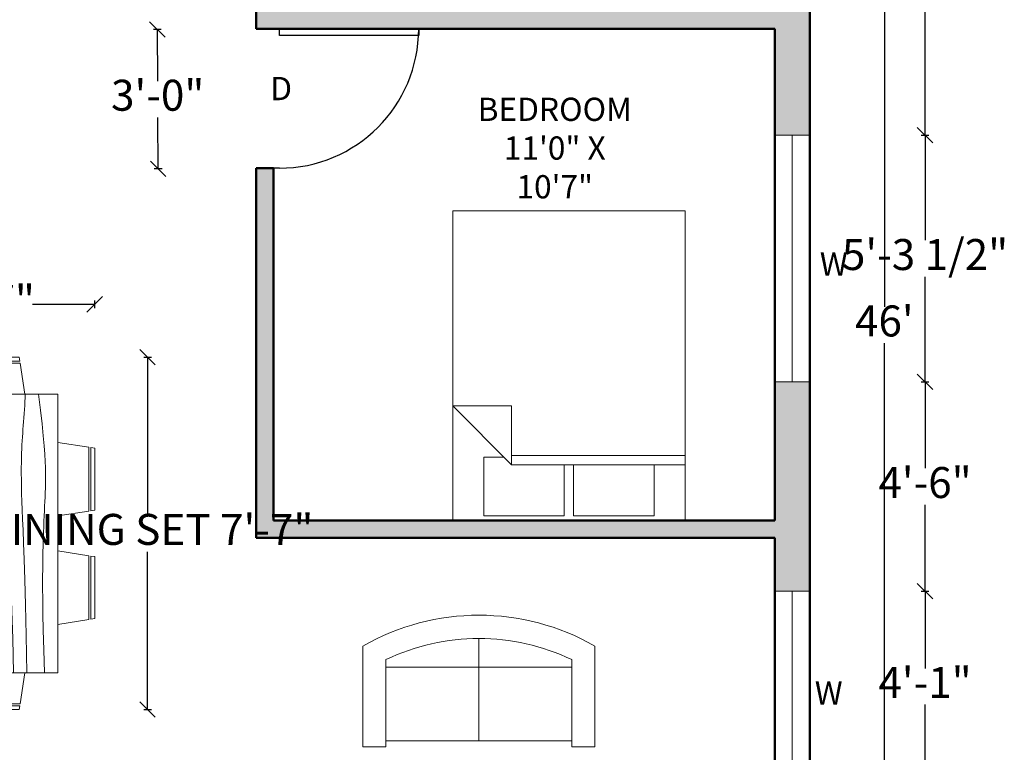
# Model space of a CAD drawing. Units: inches. Extents: x 2395 to 2921, y 528 to 1164.
# Tile 4 of 5: x 2662 to 2916, y 735 to 925. Entities that reach past the tile are written whole.
import ezdxf

# ---------------------------------------------------------------- set-up
doc = ezdxf.new("R2010")
doc.units = ezdxf.units.IN
for name, color, linetype, lineweight in [('A-ANNO-DIMS', 2, 'Continuous', 18), ('A-ANNO-TEXT', 7, 'Continuous', 18), ('A-AREA-IDEN', 7, 'Continuous', 25), ('A-DOOR', 3, 'Continuous', 25), ('A-FURN', 8, 'Continuous', 18), ('A-GLAZ', 4, 'Continuous', 18), ('A-WALL', 162, 'Continuous', 50), ('A-WALL-PATT', 162, 'Continuous', 13)]:
    doc.layers.add(name, color=color, linetype=linetype, lineweight=lineweight)
doc.styles.get("Standard").update_dxf_attribs({"font": 'arial.ttf'})
doc.dimstyles.new('ISO-25', dxfattribs={"dimtxt": 8, "dimasz": 4, "dimexe": 1, "dimexo": 1, "dimtad": 0, "dimtih": 1, "dimtoh": 1, "dimlunit": 3, "dimtxsty": 'Standard', "dimblk": 'OBLIQUE', "dimcen": 2.5, "dimadec": 0, "dimazin": 0, "dimtfac": 1, "dimtmove": 0, "dimatfit": 3, "dimfxl": 1, "dimfxlon": 1, "dimarcsym": 0})

# ---------------------------------------------------------------- blocks, each defined once
blk = doc.blocks.new('*U7')
for p, q in [((0, 0), (0, -6)), ((36, 0), (36, -6))]:
    blk.add_line(p, q)
blk.add_lwpolyline([(0, 0), (0, 36), (1.75, 36), (1.75, 0)], close=True)
blk.add_arc((0, 0), 36, 0, 90)
blk = doc.blocks.new('Sofa - Roundback Loveseat 5 ft.')
for p, q in [((0, -32.44198), (0, -5.99998)), ((-24, -33.99998), (-24, -11.46958)), ((24.00004, -33.99998), (24.00004, -11.46958)), ((-23.9998, -13.38178), (23.99986, -13.38178)), ((-24, -32.44198), (24.00004, -32.44198))]:
    blk.add_line(p, q)
for points in [[(-24, -33.99998), (-30, -33.99998), (-30, -7.99998)], [(30.00004, -7.99998), (30.00004, -33.99998), (24.00004, -33.99998)]]:
    blk.add_lwpolyline(points)
for centre, radius, start, end in [((0, -60.24998), 60.24998, 60.13715, 119.8628), ((0, -61.38438), 55.38444, 64.32083, 115.6792)]:
    blk.add_arc(centre, radius, start, end)
blk = doc.blocks.new('Dining Set - 36 x 72 in.')
for p, q in [((-22.2343, 26.00059), (-23.4847, 17.99762)), ((-22.2304, 26), (-5.7608, 26)), ((-22, 27.5), (-22.1562, 26.50042)), ((-5.8416, 26.5), (-22.1534, 26.5)), ((-22, 27.5), (-6, 27.5)), ((-5.8437, 26.49966), (-6, 27.5)), ((-4.5152, 17.99762), (-5.7655, 25.99926)), ((5.7657, 26.00059), (4.5153, 17.99762)), ((5.7696, 26), (22.2392, 26)), ((6, 27.5), (5.8438, 26.50042)), ((22.1584, 26.5), (5.8466, 26.5)), ((6, 27.5), (22, 27.5)), ((22.1563, 26.49966), (22, 27.5)), ((23.4848, 17.99762), (22.2345, 25.99926)), ((36, 18), (-36, 18)), ((-36, 18), (-36, -18)), ((36, -18), (36, 18)), ((-45.5, 8), (-44.5004, 8.15617)), ((-45.5, 8), (-45.5, -8)), ((-44.5, -8.15843), (-44.5, 8.15338)), ((-44.0006, 8.23428), (-35.9976, 9.48474)), ((-44, 8.23041), (-44, -8.23915)), ((44.0006, 8.23428), (35.9976, 9.48474)), ((44, 8.23041), (44, -8.23915)), ((44.5, -8.15843), (44.5, 8.15338)), ((45.5, 8), (44.5005, 8.15617)), ((45.5, 8), (45.5, -8)), ((-44.4997, -8.15631), (-45.5, -8)), ((-35.9976, -9.48476), (-43.9993, -8.2345)), ((35.9976, -9.48476), (43.9993, -8.2345)), ((44.4997, -8.15631), (45.5, -8)), ((-36, -18), (36, -18)), ((-22.2343, -26.0006), (-23.4847, -17.99762)), ((-4.5152, -17.99762), (-5.7655, -25.99928)), ((5.7657, -26.0006), (4.5153, -17.99762)), ((23.4848, -17.99762), (22.2345, -25.99928)), ((-22.2304, -26), (-5.7608, -26)), ((-22, -27.5), (-22.1562, -26.50044)), ((-5.8416, -26.5), (-22.1534, -26.5)), ((-22, -27.5), (-6, -27.5)), ((-5.8437, -26.49967), (-6, -27.5)), ((5.7696, -26), (22.2392, -26)), ((6, -27.5), (5.8438, -26.50044)), ((22.1584, -26.5), (5.8466, -26.5)), ((6, -27.5), (22, -27.5)), ((22.1563, -26.49967), (22, -27.5))]:
    blk.add_line(p, q)
for points in [[(-36, 15), (-31.1772, 14.97754), (-26.8079, 14.91406), (-22.8538, 14.81543), (-19.276, 14.6875), (-16.0362, 14.53613), (-13.0957, 14.36718), (-10.4159, 14.18652), (-7.9583, 14), (-5.6904, 13.81315), (-3.6035, 13.63021), (-1.6954, 13.45508), (0.0365, 13.29166), (1.5945, 13.14388), (2.9811, 13.01562), (4.1988, 12.9108), (5.25, 12.83333), (6.1393, 12.78613), (6.8802, 12.76823), (7.4883, 12.77767), (7.9792, 12.8125), (8.3685, 12.87077), (8.6719, 12.95052), (8.9049, 13.0498), (9.0833, 13.16666), (9.2205, 13.29899), (9.3216, 13.44401), (9.3895, 13.59879), (9.4271, 13.76041), (9.4373, 13.92594), (9.4232, 14.09245), (9.3875, 14.257), (9.3333, 14.41666), (9.2638, 14.56917), (9.1836, 14.71484), (9.0975, 14.85465), (9.0104, 14.98958), (8.9272, 15.1206), (8.8529, 15.2487), (8.7922, 15.37483), (8.75, 15.5), (8.7305, 15.62467), (8.7344, 15.74739), (8.7617, 15.86621), (8.8125, 15.97916), (8.8867, 16.08431), (8.9844, 16.17968), (9.1055, 16.26334), (9.25, 16.33333), (9.4189, 16.38802), (9.6172, 16.42708), (9.8506, 16.45052), (10.125, 16.45833), (10.4463, 16.45052), (10.8203, 16.42708), (11.2529, 16.38802), (11.75, 16.33333), (12.3184, 16.26318), (12.9694, 16.17838), (13.7151, 16.07991), (14.5677, 15.96875), (15.5395, 15.84586), (16.6426, 15.71224), (17.8893, 15.56884), (19.2917, 15.41666), (20.859, 15.25667), (22.5879, 15.08984), (24.4721, 14.91715), (26.5052, 14.73958), (28.6809, 14.5581), (30.9929, 14.3737), (33.4347, 14.18733), (36, 14)], [(-36, 10), (-28.9766, 10.14274), (-23.1725, 10.20442), (-18.4241, 10.19775), (-14.5677, 10.13541), (-11.4399, 10.03011), (-8.877, 9.89453), (-6.7154, 9.74137), (-4.7917, 9.58333), (-2.9698, 9.43082), (-1.2246, 9.28515), (0.4415, 9.14534), (2.026, 9.01041), (3.5266, 8.87939), (4.9408, 8.7513), (6.266, 8.62516), (7.5, 8.5), (8.6411, 8.37549), (9.6914, 8.2539), (10.6538, 8.13818), (11.5312, 8.03125), (12.3267, 7.93603), (13.043, 7.85547), (13.6831, 7.79248), (14.25, 7.75), (14.7471, 7.7303), (15.1797, 7.73307), (15.5537, 7.75732), (15.875, 7.80208), (16.1494, 7.86637), (16.3828, 7.94922), (16.5811, 8.04964), (16.75, 8.16666), (16.8944, 8.29915), (17.0143, 8.44531), (17.1089, 8.60319), (17.1771, 8.77083), (17.218, 8.94629), (17.2305, 9.1276), (17.2137, 9.31282), (17.1667, 9.5), (17.0895, 9.6875), (16.987, 9.875), (16.8649, 10.0625), (16.7292, 10.25), (16.5856, 10.4375), (16.4401, 10.625), (16.2985, 10.8125), (16.1667, 11), (16.05, 11.18733), (15.9518, 11.3737), (15.8752, 11.5581), (15.8229, 11.73958), (15.798, 11.91715), (15.8034, 12.08984), (15.842, 12.25667), (15.9167, 12.41666), (16.0295, 12.56836), (16.1784, 12.70833), (16.3605, 12.83268), (16.5729, 12.9375), (16.8127, 13.01888), (17.0768, 13.07291), (17.3625, 13.0957), (17.6667, 13.08333), (17.9894, 13.03312), (18.3418, 12.94726), (18.7382, 12.82918), (19.1927, 12.68229), (19.7195, 12.51001), (20.3327, 12.31575), (21.0465, 12.10294), (21.875, 11.875), (22.8357, 11.63354), (23.959, 11.37304), (25.2786, 11.08618), (26.8282, 10.76562), (28.6414, 10.40405), (30.752, 9.99414), (33.1936, 9.52856), (36, 9)], [(-36, 5.5), (-30.7157, 5.3348), (-26.069, 5.20963), (-21.9946, 5.11767), (-18.4271, 5.05208), (-15.3009, 5.00602), (-12.5508, 4.97265), (-10.1112, 4.94515), (-7.9167, 4.91666), (-5.909, 4.88167), (-4.0586, 4.83984), (-2.3429, 4.79215), (-0.7396, 4.73958), (0.7739, 4.6831), (2.22, 4.6237), (3.6213, 4.56233), (5, 4.5), (6.373, 4.43782), (7.7344, 4.3776), (9.0723, 4.32129), (10.375, 4.27083), (11.6309, 4.22819), (12.8281, 4.19531), (13.9551, 4.17415), (15, 4.16666), (15.954, 4.17448), (16.819, 4.19791), (17.6001, 4.23698), (18.3021, 4.29166), (18.9299, 4.36198), (19.4883, 4.44791), (19.9823, 4.54948), (20.4167, 4.66666), (20.7969, 4.79899), (21.1302, 4.94401), (21.4245, 5.09879), (21.6875, 5.26041), (21.9271, 5.42594), (22.1511, 5.59245), (22.3672, 5.757), (22.5834, 5.91666), (22.8065, 6.06868), (23.0404, 6.21093), (23.2879, 6.34147), (23.5521, 6.45833), (23.8358, 6.55957), (24.142, 6.64323), (24.4735, 6.70735), (24.8334, 6.75), (25.2235, 6.76969), (25.642, 6.76692), (26.0858, 6.74267), (26.5521, 6.69791), (27.0379, 6.63362), (27.5404, 6.55078), (28.0565, 6.45036), (28.5834, 6.33333), (29.1242, 6.19987), (29.7071, 6.04687), (30.3661, 5.87044), (31.1354, 5.66666), (32.0493, 5.43164), (33.142, 5.16146), (34.4475, 4.85221), (36, 4.5)], [(-36, -1), (-30.7915, -0.6591), (-26.0195, -0.38216), (-21.6519, -0.16284), (-17.6563, 0.00521), (-14.0005, 0.12833), (-10.6523, 0.21289), (-7.5796, 0.26522), (-4.75, 0.29166), (-2.134, 0.29793), (0.2878, 0.28711), (2.5317, 0.26163), (4.6146, 0.22396), (6.5529, 0.17651), (8.3633, 0.12174), (10.0623, 0.06209), (11.6667, 0), (13.1899, -0.06201), (14.6341, -0.1211), (15.9982, -0.17432), (17.2813, -0.21875), (18.4823, -0.25147), (19.6003, -0.26953), (20.6343, -0.27002), (21.5834, -0.25), (22.4481, -0.20768), (23.2357, -0.14584), (23.9549, -0.06836), (24.6146, 0.02083), (25.2235, 0.11784), (25.7904, 0.21875), (26.3241, 0.31966), (26.8334, 0.41666), (27.3265, 0.50618), (27.8099, 0.58593), (28.2894, 0.65397), (28.7709, 0.70833), (29.2601, 0.74707), (29.763, 0.76823), (30.2855, 0.76985), (30.8334, 0.75), (31.4088, 0.70784), (31.9994, 0.64713), (32.589, 0.57275), (33.1615, 0.48958), (33.7008, 0.4025), (34.1908, 0.3164), (34.6153, 0.23616), (34.9584, 0.16666), (35.2099, 0.11165), (35.3848, 0.07031), (35.504, 0.04069), (35.5886, 0.02083), (35.6594, 0.00879), (35.7377, 0.0026), (35.8442, 0.00032), (36, 0)], [(-36, -6.5), (-27.1843, -6.31267), (-20.084, -6.1263), (-14.469, -5.9419), (-10.1094, -5.76042), (-6.7752, -5.58285), (-4.2363, -5.41016), (-2.2629, -5.24333), (-0.625, -5.08334), (0.8708, -4.93099), (2.2715, -4.78646), (3.5872, -4.64974), (4.8281, -4.52084), (6.0046, -4.39974), (7.127, -4.28646), (8.2053, -4.18099), (9.25, -4.08334), (10.2705, -3.99382), (11.2734, -3.91407), (12.2647, -3.84603), (13.25, -3.79167), (14.2354, -3.75293), (15.2266, -3.73177), (16.2295, -3.73015), (17.25, -3.75), (18.2912, -3.79248), (19.3451, -3.85547), (20.4009, -3.93604), (21.4479, -4.03125), (22.4754, -4.13819), (23.4727, -4.25391), (24.4289, -4.37549), (25.3334, -4.5), (26.1785, -4.62492), (26.9694, -4.74935), (27.7145, -4.87281), (28.4219, -4.99479), (29.1, -5.11483), (29.7572, -5.23242), (30.4016, -5.34709), (31.0417, -5.45834), (31.6837, -5.56437), (32.3262, -5.65821), (32.9658, -5.73153), (33.599, -5.77604), (34.2224, -5.78345), (34.8327, -5.74545), (35.4264, -5.65373), (36, -5.5)], [(-36, -10), (-26.4022, -9.81299), (-18.4675, -9.62891), (-11.9839, -9.45069), (-6.7396, -9.28125), (-2.5226, -9.12354), (0.8789, -8.98047), (3.6769, -8.85498), (6.0833, -8.75), (8.2767, -8.66765), (10.3021, -8.60677), (12.1712, -8.56543), (13.8958, -8.54167), (15.4876, -8.53353), (16.9583, -8.53907), (18.3197, -8.55632), (19.5834, -8.58334), (20.7616, -8.61841), (21.8685, -8.66081), (22.9188, -8.71004), (23.9271, -8.76563), (24.9081, -8.82707), (25.8763, -8.89388), (26.8465, -8.96558), (27.8334, -9.04167), (28.8474, -9.12118), (29.8828, -9.20117), (30.93, -9.27824), (31.9792, -9.34896), (33.0205, -9.40991), (34.0443, -9.45768), (35.0407, -9.48885), (36, -9.5)], [(-36, -14.5), (-30.0881, -14.33513), (-25.0332, -14.21224), (-20.7312, -14.12647), (-17.0781, -14.07292), (-13.97, -14.04671), (-11.3027, -14.04297), (-8.9724, -14.05681), (-6.875, -14.08334), (-4.9224, -14.11833), (-3.0905, -14.16016), (-1.3709, -14.20785), (0.2448, -14.26042), (1.7647, -14.3169), (3.1973, -14.3763), (4.5507, -14.43767), (5.8333, -14.5), (7.0554, -14.5621), (8.235, -14.62175), (9.3922, -14.67652), (10.5469, -14.72396), (11.7192, -14.76164), (12.929, -14.78711), (14.1965, -14.79794), (15.5417, -14.79167), (16.9933, -14.76424), (18.6152, -14.70508), (20.4804, -14.60197), (22.6615, -14.44271), (25.2312, -14.21509), (28.2624, -13.9069), (31.8277, -13.50594), (36, -13)]]:
    blk.add_lwpolyline(points)
blk = doc.blocks.new('Bed - Queen')
for p, q in [((0, -80.00003), (0, 0)), ((0, 0), (59.99999, 0)), ((59.99999, 0), (59.99999, -80.00003)), ((7.99999, -1.2), (28.79998, -1.2)), ((7.99999, -14.4), (7.99999, -1.2)), ((28.79998, -1.2), (28.79998, -14.4)), ((31.19999, -1.2), (51.99999, -1.2)), ((31.19999, -14.4), (31.19999, -1.2)), ((51.99999, -1.2), (51.99999, -16.4)), ((0, -14.4), (44.8, -14.4)), ((59.99999, -29.6), (44.8, -14.4)), ((44.8, -14.4), (44.8, -29.6)), ((44.8, -16.8), (0, -16.8)), ((51.99999, -16.4), (46.79936, -16.4)), ((44.8, -29.6), (59.99999, -29.6)), ((59.99999, -80.00003), (0, -80.00003))]:
    blk.add_line(p, q)
blk = doc.blocks.new('_Oblique')
at = {"color": 0, "linetype": 'ByBlock', "lineweight": -2}
blk.add_line((-0.5, -0.5), (0.5, 0.5), dxfattribs=at)
blk = doc.blocks.new('*D20')
at = {"layer": 'A-ANNO-DIMS', "color": 0, "lineweight": -2, "transparency": 16777216}
for p, q in [((2884.49, 1121.85), (2886.49, 1121.85)), ((2885.49, 1121.85), (2885.49, 850.56)), ((2885.49, 569.85), (2885.49, 841.14)), ((2884.49, 569.85), (2886.49, 569.85))]:
    blk.add_line(p, q, dxfattribs=at)
at = {"layer": 'Defpoints', "color": 0, "transparency": 16777216}
for p in [(2866.2, 1121.85), (2866.2, 569.85), (2885.49, 569.85)]:
    blk.add_point(p, dxfattribs=at)
at = {"layer": 'A-ANNO-DIMS', "color": 0, "lineweight": -2, "transparency": 16777216, "xscale": 4, "yscale": 4, "zscale": 4}
for p, rotation in [((2885.49, 1121.85), 90), ((2885.49, 569.85), 270)]:
    blk.add_blockref('_Oblique', p, dxfattribs=dict(at, rotation=rotation))
at = {"layer": 'A-ANNO-DIMS', "color": 0, "transparency": 16777216, "insert": (2885.49, 845.85), "char_height": 8, "attachment_point": 5}
blk.add_mtext("46'", dxfattribs=at)
blk = doc.blocks.new('*D36')
at = {"layer": 'A-ANNO-DIMS', "color": 0, "lineweight": -2, "transparency": 16777216}
for p, q in [((2694.16, 837.52), (2696.16, 837.52)), ((2695.16, 837.52), (2695.16, 796.78)), ((2695.16, 746.52), (2695.16, 787.26)), ((2694.16, 746.52), (2696.16, 746.52))]:
    blk.add_line(p, q, dxfattribs=at)
at = {"layer": 'Defpoints', "color": 0, "transparency": 16777216}
for p in [(2681.51, 837.52), (2695.16, 837.52), (2681.51, 746.52)]:
    blk.add_point(p, dxfattribs=at)
at = {"layer": 'A-ANNO-DIMS', "color": 0, "lineweight": -2, "transparency": 16777216, "xscale": 4, "yscale": 4, "zscale": 4}
for p, rotation in [((2695.16, 837.52), 90), ((2695.16, 746.52), 270)]:
    blk.add_blockref('_Oblique', p, dxfattribs=dict(at, rotation=rotation))
at = {"layer": 'A-ANNO-DIMS', "color": 0, "transparency": 16777216, "insert": (2695.16, 792.02), "char_height": 8, "attachment_point": 5}
blk.add_mtext('DINING SET 7\'-7"', dxfattribs=at)
blk = doc.blocks.new('*D37')
at = {"layer": 'A-ANNO-DIMS', "color": 0, "lineweight": -2, "transparency": 16777216}
for p, q in [((2626.51, 850.17), (2626.51, 852.17)), ((2681.51, 850.17), (2681.51, 852.17)), ((2626.51, 851.17), (2642.59, 851.17)), ((2681.51, 851.17), (2665.43, 851.17))]:
    blk.add_line(p, q, dxfattribs=at)
at = {"layer": 'Defpoints', "color": 0, "transparency": 16777216}
for p in [(2626.51, 851.17), (2626.51, 837.52), (2681.51, 837.52)]:
    blk.add_point(p, dxfattribs=at)
at = {"layer": 'A-ANNO-DIMS', "color": 0, "lineweight": -2, "transparency": 16777216, "xscale": 4, "yscale": 4, "zscale": 4, "rotation": 180}
blk.add_blockref('_Oblique', (2626.51, 851.17), dxfattribs=at)
at = {"layer": 'A-ANNO-DIMS', "color": 0, "lineweight": -2, "transparency": 16777216, "xscale": 4, "yscale": 4, "zscale": 4}
blk.add_blockref('_Oblique', (2681.51, 851.17), dxfattribs=at)
at = {"layer": 'A-ANNO-DIMS', "color": 0, "transparency": 16777216, "insert": (2654.01, 851.17), "char_height": 8, "attachment_point": 5}
blk.add_mtext('4\'-7"', dxfattribs=at)
blk = doc.blocks.new('*D65')
at = {"layer": 'A-ANNO-DIMS', "color": 0, "lineweight": -2, "transparency": 16777216}
for p, q in [((2895, 777.1), (2897, 777.1)), ((2896, 777.1), (2896, 757.14)), ((2896, 727.91), (2896, 747.86)), ((2895, 727.91), (2897, 727.91))]:
    blk.add_line(p, q, dxfattribs=at)
at = {"layer": 'Defpoints', "color": 0, "transparency": 16777216}
for p in [(2866.2, 777.1), (2896, 777.1), (2866.2, 727.91)]:
    blk.add_point(p, dxfattribs=at)
at = {"layer": 'A-ANNO-DIMS', "color": 0, "lineweight": -2, "transparency": 16777216, "xscale": 4, "yscale": 4, "zscale": 4}
for p, rotation in [((2896, 777.1), 90), ((2896, 727.91), 270)]:
    blk.add_blockref('_Oblique', p, dxfattribs=dict(at, rotation=rotation))
at = {"layer": 'A-ANNO-DIMS', "color": 0, "transparency": 16777216, "insert": (2896, 752.5), "char_height": 8, "attachment_point": 5}
blk.add_mtext('4\'-1"', dxfattribs=at)
blk = doc.blocks.new('*D66')
at = {"layer": 'A-ANNO-DIMS', "color": 0, "lineweight": -2, "transparency": 16777216}
for p, q in [((2895, 831.15), (2897, 831.15)), ((2896, 831.15), (2896, 808.83)), ((2896, 777.1), (2896, 799.42)), ((2895, 777.1), (2897, 777.1))]:
    blk.add_line(p, q, dxfattribs=at)
at = {"layer": 'Defpoints', "color": 0, "transparency": 16777216}
for p in [(2866.2, 831.15), (2896, 831.15), (2866.2, 777.1)]:
    blk.add_point(p, dxfattribs=at)
at = {"layer": 'A-ANNO-DIMS', "color": 0, "lineweight": -2, "transparency": 16777216, "xscale": 4, "yscale": 4, "zscale": 4}
for p, rotation in [((2896, 831.15), 90), ((2896, 777.1), 270)]:
    blk.add_blockref('_Oblique', p, dxfattribs=dict(at, rotation=rotation))
at = {"layer": 'A-ANNO-DIMS', "color": 0, "transparency": 16777216, "insert": (2896, 804.12), "char_height": 8, "attachment_point": 5}
blk.add_mtext('4\'-6"', dxfattribs=at)
blk = doc.blocks.new('*D67')
at = {"layer": 'A-ANNO-DIMS', "color": 0, "lineweight": -2, "transparency": 16777216}
for p, q in [((2895, 894.87), (2897, 894.87)), ((2896, 894.87), (2896, 867.78)), ((2896, 831.15), (2896, 858.25)), ((2895, 831.15), (2897, 831.15))]:
    blk.add_line(p, q, dxfattribs=at)
at = {"layer": 'Defpoints', "color": 0, "transparency": 16777216}
for p in [(2866.2, 894.87), (2896, 894.87), (2866.2, 831.15)]:
    blk.add_point(p, dxfattribs=at)
at = {"layer": 'A-ANNO-DIMS', "color": 0, "lineweight": -2, "transparency": 16777216, "xscale": 4, "yscale": 4, "zscale": 4}
for p, rotation in [((2896, 894.87), 90), ((2896, 831.15), 270)]:
    blk.add_blockref('_Oblique', p, dxfattribs=dict(at, rotation=rotation))
at = {"layer": 'A-ANNO-DIMS', "color": 0, "transparency": 16777216, "insert": (2896, 863.01), "char_height": 8, "attachment_point": 5}
blk.add_mtext('5\'-3 1/2"', dxfattribs=at)
blk = doc.blocks.new('*D68')
at = {"layer": 'A-ANNO-DIMS', "color": 0, "lineweight": -2, "transparency": 16777216}
for p, q in [((2895, 985.13), (2897, 985.13)), ((2896, 985.13), (2896, 944.76)), ((2896, 894.87), (2896, 935.24)), ((2895, 894.87), (2897, 894.87))]:
    blk.add_line(p, q, dxfattribs=at)
at = {"layer": 'Defpoints', "color": 0, "transparency": 16777216}
for p in [(2866.2, 985.13), (2896, 985.13), (2866.2, 894.87)]:
    blk.add_point(p, dxfattribs=at)
at = {"layer": 'A-ANNO-DIMS', "color": 0, "lineweight": -2, "transparency": 16777216, "xscale": 4, "yscale": 4, "zscale": 4}
for p, rotation in [((2896, 985.13), 90), ((2896, 894.87), 270)]:
    blk.add_blockref('_Oblique', p, dxfattribs=dict(at, rotation=rotation))
at = {"layer": 'A-ANNO-DIMS', "color": 0, "transparency": 16777216, "insert": (2896, 940), "char_height": 8, "attachment_point": 5}
blk.add_mtext('7\'-6 1/2"', dxfattribs=at)
blk = doc.blocks.new('*D73')
at = {"layer": 'A-ANNO-DIMS', "color": 0, "lineweight": -2, "transparency": 16777216}
for p, q in [((2669.2, 541.05), (2669.2, 539.05)), ((2669.2, 540.05), (2672.87, 540.05)), ((2699.2, 540.05), (2695.53, 540.05)), ((2699.2, 541.05), (2699.2, 539.05))]:
    blk.add_line(p, q, dxfattribs=at)
at = {"layer": 'Defpoints', "color": 0, "transparency": 16777216}
for p in [(2669.2, 988.35), (2699.2, 988.35), (2699.2, 540.05)]:
    blk.add_point(p, dxfattribs=at)
at = {"layer": 'A-ANNO-DIMS', "color": 0, "lineweight": -2, "transparency": 16777216, "xscale": 4, "yscale": 4, "zscale": 4, "rotation": 180}
blk.add_blockref('_Oblique', (2669.2, 540.05), dxfattribs=at)
at = {"layer": 'A-ANNO-DIMS', "color": 0, "lineweight": -2, "transparency": 16777216, "xscale": 4, "yscale": 4, "zscale": 4}
blk.add_blockref('_Oblique', (2699.2, 540.05), dxfattribs=at)
at = {"layer": 'A-ANNO-DIMS', "color": 0, "transparency": 16777216, "insert": (2684.2, 540.05), "char_height": 8, "attachment_point": 5}
blk.add_mtext('2\'-6"', dxfattribs=at)
blk = doc.blocks.new('*D76')
at = {"layer": 'A-ANNO-DIMS', "color": 0, "lineweight": -2, "transparency": 16777216}
for p, q in [((2698.65, 922.15), (2696.65, 922.14)), ((2697.65, 922.15), (2697.74, 908.86)), ((2697.9, 886.15), (2697.81, 899.43)), ((2698.9, 886.15), (2696.9, 886.14))]:
    blk.add_line(p, q, dxfattribs=at)
at = {"layer": 'Defpoints', "color": 0, "transparency": 16777216}
for p in [(2697.65, 922.15), (2727.45, 922.35), (2727.7, 886.35)]:
    blk.add_point(p, dxfattribs=at)
at = {"layer": 'A-ANNO-DIMS', "color": 0, "lineweight": -2, "transparency": 16777216, "xscale": 4, "yscale": 4, "zscale": 4}
for p, rotation in [((2697.65, 922.15), 90.39788096183464), ((2697.9, 886.15), 270.3978809618346)]:
    blk.add_blockref('_Oblique', p, dxfattribs=dict(at, rotation=rotation))
at = {"layer": 'A-ANNO-DIMS', "color": 0, "transparency": 16777216, "insert": (2697.78, 904.15), "char_height": 8, "attachment_point": 5}
blk.add_mtext('3\'-0"', dxfattribs=at)

msp = doc.modelspace()

# ---------------------------------------------------------------- hatches: boundary and pattern name
at = {"layer": 'A-WALL-PATT'}
h = msp.add_hatch(color=256, dxfattribs=at)
h.dxf.hatch_style = 1
h.paths.add_polyline_path([(2627.2, 1121.853), (2446.2, 1121.853), (2446.2, 1054.648), (2455.2, 1054.648), (2455.2, 1112.853), (2606.2, 1112.853), (2606.2, 1022.853), (2610.7, 1022.853), (2610.7, 1112.853), (2627.2, 1112.853)])
h.paths.add_polyline_path([(2685.7, 1121.853), (2648.2, 1121.853), (2648.2, 1112.853), (2664.7, 1112.853), (2664.7, 992.853), (2606.2, 992.853), (2606.2, 962.853), (2610.7, 962.853), (2610.7, 988.353), (2669.2, 988.353), (2669.2, 994.353), (2669.2, 1024.353), (2669.2, 1112.853), (2685.7, 1112.853)])
h.paths.add_polyline_path([(2866.2, 1121.853), (2706.7, 1121.853), (2706.7, 1112.853), (2723.2, 1112.853), (2723.2, 992.853), (2699.2, 992.853), (2699.2, 988.353), (2723.2, 988.353), (2723.2, 962.853), (2727.7, 962.853), (2727.7, 1112.853), (2857.2, 1112.853), (2857.2, 1049.508), (2866.2, 1049.508)])
h.paths.add_polyline_path([(2866.2, 985.129), (2857.2, 985.129), (2857.2, 926.853), (2723.2, 926.853), (2723.2, 922.353), (2729.2, 922.353), (2765.2, 922.353), (2857.2, 922.353), (2857.2, 894.873), (2866.2, 894.873)])
h.paths.add_polyline_path([(2455.2, 997.652), (2446.2, 997.652), (2446.2, 909.181), (2455.2, 908.938), (2455.2, 922.353), (2610.7, 922.353), (2610.7, 926.853), (2455.2, 926.853)])
h.paths.add_polyline_path([(2455.2, 838.353), (2610.7, 838.353), (2610.7, 842.853), (2455.2, 842.853), (2455.2, 856.236), (2446.2, 856.236), (2446.2, 815.427), (2455.2, 815.427)])
h.paths.add_polyline_path([(2455.2, 772.706), (2446.2, 772.706), (2446.2, 569.853), (2505.031, 569.853), (2505.031, 578.853), (2455.2, 578.853), (2455.2, 734.853), (2570.2, 734.853), (2570.2, 739.353), (2568.7, 739.353), (2568.7, 806.353), (2564.2, 806.353), (2564.2, 739.353), (2455.2, 739.353)])
h.paths.add_polyline_path([(2656.2, 578.853), (2610.7, 578.853), (2610.7, 739.353), (2606.2, 739.353), (2606.2, 578.853), (2565.031, 578.853), (2565.031, 569.853), (2656.2, 569.853)])
h.paths.add_polyline_path([(2733.198, 578.853), (2716.2, 578.853), (2716.2, 569.853), (2733.198, 569.853)])
h.paths.add_polyline_path([(2801.188, 578.853), (2764.893, 578.853), (2764.893, 569.853), (2801.188, 569.853)])
h.paths.add_polyline_path([(2866.2, 616.306), (2857.2, 616.306), (2857.2, 578.853), (2836.314, 578.853), (2836.314, 569.853), (2866.2, 569.853)])
h.paths.add_polyline_path([(2866.2, 727.906), (2857.2, 727.906), (2857.2, 670.095), (2866.2, 670.095)])
h.paths.add_polyline_path([(2866.2, 831.149), (2857.2, 831.149), (2857.2, 795.353), (2727.7, 795.353), (2727.7, 886.353), (2723.2, 886.353), (2723.2, 790.853), (2857.2, 790.853), (2857.2, 777.101), (2866.2, 777.101)])

# ---------------------------------------------------------------- linework, layer by layer
at = {"layer": 'A-GLAZ'}
for p, q in [((2857.2, 894.873), (2866.2, 894.873)), ((2861.7, 831.149), (2861.7, 894.873)), ((2857.2, 831.149), (2866.2, 831.149)), ((2857.2, 777.101), (2866.2, 777.101)), ((2861.7, 727.906), (2861.7, 777.101))]:
    msp.add_line(p, q, dxfattribs=at)
at = {"layer": 'A-WALL'}
for p, q in [((2866.2, 569.853), (2866.2, 1121.853)), ((2723.2, 926.853), (2723.2, 922.353)), ((2857.2, 922.353), (2723.2, 922.353)), ((2857.2, 795.353), (2857.2, 922.353)), ((2723.2, 886.353), (2723.2, 790.853)), ((2723.2, 886.353), (2727.7, 886.353)), ((2727.7, 886.353), (2727.7, 795.353)), ((2857.2, 795.353), (2727.7, 795.353)), ((2857.2, 790.853), (2723.2, 790.853)), ((2857.2, 578.853), (2857.2, 790.853))]:
    msp.add_line(p, q, dxfattribs=at)

# ---------------------------------------------------------------- block references
at = {"layer": 'A-DOOR', "rotation": 270}
msp.add_blockref('*U7', (2729.2, 922.353), dxfattribs=at)
at = {"layer": 'A-FURN'}
for name, p, rotation in [('Bed - Queen', (2833.995, 795.353), 180), ('Dining Set - 36 x 72 in.', (2654.008, 792.019), 90)]:
    msp.add_blockref(name, p, dxfattribs=dict(at, rotation=rotation))
msp.add_blockref('Sofa - Roundback Loveseat 5 ft.', (2780.741, 770.892), dxfattribs=at)

# ---------------------------------------------------------------- texts
at = {"layer": 'A-ANNO-TEXT', "char_height": 6, "attachment_point": 1}
for s, insert in [('\\pxqc;D', (2723.454, 909.91)), ('\\pxqc;W', (2866.2, 864.587)), ('\\pxqc;W', (2864.903, 753.807))]:
    msp.add_mtext_dynamic_manual_height_columns(s, width=12.42697, gutter_width=12.5, heights=[0], dxfattribs=dict(at, insert=insert))
at = {"layer": 'A-AREA-IDEN', "insert": (2780.356, 904.553), "char_height": 6, "attachment_point": 1}
msp.add_mtext_dynamic_manual_height_columns('\\pxqc;BEDROOM\\P11\'0" X 10\'7"', width=39.98375, gutter_width=12.5, heights=[0], dxfattribs=at)

# ---------------------------------------------------------------- dimensions: what is measured, and where the dimension line sits
at = {"layer": 'A-ANNO-DIMS'}
for base, p1, p2, angle, override, picture, middle in [((2885.489, 569.853), (2866.2, 1121.853), (2866.2, 569.853), 90, {"dimclrd": 0, "dimclre": 0, "dimclrt": 0}, '*D20', (2885.489, 845.853)), ((2896, 985.129), (2866.2, 894.873), (2866.2, 985.129), 90, {"dimdec": 1, "dimlfac": 1, "dimrnd": 0, "dimzin": 1, "dimdsep": 46, "dimlunit": 4, "dimfrac": 2}, '*D68', (2896, 940.001)), ((2697.651, 922.146), (2727.7, 886.353), (2727.45, 922.353), 90.39788, {"dimdec": 1, "dimlfac": 1, "dimrnd": 0, "dimzin": 1, "dimdsep": 46, "dimlunit": 4, "dimfrac": 2}, '*D76', (2697.776, 904.146)), ((2896, 894.873), (2866.2, 831.149), (2866.2, 894.873), 90, {"dimdec": 1, "dimlfac": 1, "dimrnd": 0, "dimzin": 1, "dimdsep": 46, "dimlunit": 4, "dimfrac": 2}, '*D67', (2896, 863.011)), ((2626.508, 851.169), (2681.508, 837.519), (2626.508, 837.519), 180, {"dimdec": 1, "dimlfac": 1, "dimrnd": 0, "dimzin": 1, "dimdsep": 46, "dimlunit": 4, "dimfrac": 2}, '*D37', (2654.008, 851.169)), ((2896, 831.149), (2866.2, 777.101), (2866.2, 831.149), 90, {"dimdec": 1, "dimlfac": 1, "dimrnd": 0, "dimzin": 1, "dimdsep": 46, "dimlunit": 4, "dimfrac": 2}, '*D66', (2896, 804.125)), ((2896, 777.101), (2866.2, 727.906), (2866.2, 777.101), 90, {"dimdec": 1, "dimlfac": 1, "dimrnd": 0, "dimzin": 1, "dimdsep": 46, "dimlunit": 4, "dimfrac": 2}, '*D65', (2896, 752.503))]:
    dim = msp.add_linear_dim(base=base, p1=p1, p2=p2, angle=angle, dimstyle='ISO-25', override=override, dxfattribs=at)
    dim.commit()
    dim.dimension.update_dxf_attribs({"geometry": picture, "text_midpoint": middle})
dim = msp.add_linear_dim(base=(2699.2, 540.053), p1=(2669.2, 988.353), p2=(2699.2, 988.353), dimstyle='ISO-25', override={"dimdec": 1, "dimlfac": 1, "dimrnd": 0, "dimzin": 1, "dimdsep": 46, "dimlunit": 4, "dimfrac": 2}, dxfattribs=at)
dim.commit()
dim.dimension.update_dxf_attribs({"geometry": '*D73', "text_midpoint": (2684.2, 540.053)})
dim = msp.add_linear_dim(base=(2695.158, 837.519), p1=(2681.508, 746.519), p2=(2681.508, 837.519), angle=90, text='DINING SET <>', dimstyle='ISO-25', override={"dimdec": 1, "dimlfac": 1, "dimrnd": 0, "dimzin": 1, "dimdsep": 46, "dimlunit": 4, "dimfrac": 2}, dxfattribs=at)
dim.commit()
dim.dimension.update_dxf_attribs({"geometry": '*D36', "text_midpoint": (2695.158, 792.019)})

doc.saveas('drawing.dxf')
